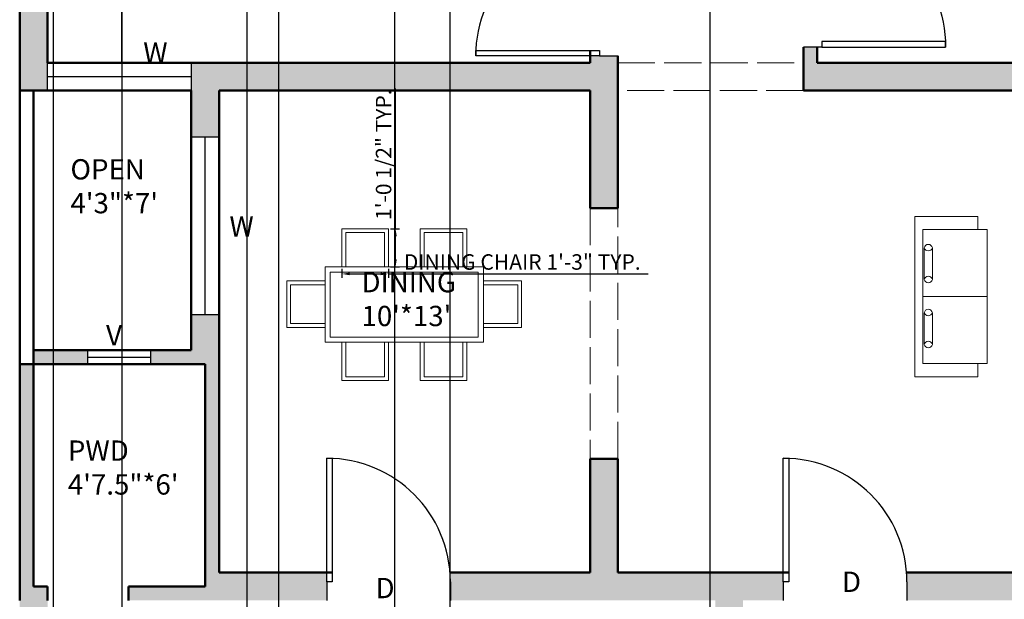
# Model space of a CAD drawing. Units: inches. Extents: x 2101 to 2663, y 1144 to 2069.
# Tile 2 of 4: x 2112 to 2431, y 1530 to 1718. Entities that reach past the tile are written whole.
import ezdxf

# ---------------------------------------------------------------- set-up
doc = ezdxf.new("R2010")
doc.units = ezdxf.units.IN
doc.linetypes.add('ACAD_ISO02W100', pattern=[15, 12, -3])
for name, color, linetype, lineweight in [('A-ANNO-DIMS', 2, 'Continuous', 18), ('A-ANNO-TEXT', 7, 'Continuous', 18), ('A-AREA-IDEN', 7, 'Continuous', 25), ('A-FLOR-CASE', 142, 'Continuous', 25), ('A-WALL-OVHD', 240, 'ACAD_ISO02W100', 18), ('A-WALL-PATT', 240, 'Continuous', 13), ('door', 52, 'Continuous', 25), ('fur', 142, 'Continuous', 18), ('wall', 240, 'Continuous', 50), ('win', 150, 'Continuous', 25)]:
    doc.layers.add(name, color=color, linetype=linetype, lineweight=lineweight)
doc.styles.get("Standard").update_dxf_attribs({"font": 'arial.ttf'})
doc.dimstyles.new('ISO-25', dxfattribs={"dimtxt": 5, "dimasz": 2.5, "dimexe": 1.25, "dimexo": 0.625, "dimtad": 1, "dimdec": 0, "dimlunit": 4, "dimtxsty": 'Standard', "dimcen": 2.5, "dimadec": 0, "dimazin": 0, "dimtfac": 1, "dimtdec": 0, "dimtmove": 0, "dimatfit": 3, "dimfxl": 1, "dimarcsym": 0})

# ---------------------------------------------------------------- blocks, each defined once
blk = doc.blocks.new('*U2')
for p, q in [((0, 0), (0, -6)), ((40, 0), (40, -6))]:
    blk.add_line(p, q)
blk.add_lwpolyline([(0, 0), (0, 40), (1.75, 40), (1.75, 0)], close=True)
blk.add_arc((0, 0), 40, 0, 90)
blk = doc.blocks.new('SOFA-TWO-SEAT')
for p, q in [((-8.65, 21.68), (-8.65, 25.93)), ((-8.65, 25.93), (11.73, 25.93)), ((11.73, 25.93), (11.73, -25.93)), ((-11.73, -0.01), (9.09, -0.01)), ((-8.65, -25.93), (-8.65, -21.7)), ((11.73, -25.93), (-8.65, -25.93))]:
    blk.add_line(p, q)
blk.add_lwpolyline([(9.09, 21.68), (-11.73, 21.68), (-11.73, -21.7), (9.09, -21.7)], close=True)
for points in [[(6.04, 5.2), (6.04, 15.47)], [(8.66, 15.47), (8.66, 5.2)], [(6.04, -15.8), (6.04, -5.54)], [(8.66, -5.54), (8.66, -15.8)]]:
    blk.add_lwpolyline(points)
for centre, radius, start, end in [((7.35, 15.19), 1.34, 11.9211, 168.0789), ((7.35, 15.75), 1.34, 191.8934, 348.1066), ((7.35, 4.81), 1.37, 16.4476, 163.5524), ((7.35, 5.4), 1.33, 188.6987, 351.3013), ((7.35, -5.81), 1.34, 11.9211, 168.0789), ((7.35, -5.26), 1.34, 191.8934, 348.1066), ((7.35, -16.19), 1.37, 16.4476, 163.5524), ((7.35, -15.6), 1.33, 188.6987, 351.3013)]:
    blk.add_arc(centre, radius, start, end)
blk = doc.blocks.new('CHAIR-DINING')
for p, q in [((-7.55, -6.18), (-7.55, 6.18)), ((-7.55, 6.18), (7.55, 6.18)), ((7.55, 6.18), (7.55, -6.18))]:
    blk.add_line(p, q)
blk.add_lwpolyline([(-6.25, -6.18), (6.27, -6.18), (6.27, 5), (-6.25, 5)], close=True)
blk = doc.blocks.new('*D25')
at = {"layer": 'A-ANNO-DIMS', "color": 0, "lineweight": -2, "transparency": 16777216}
for p, q in [((2216.58, 1636.95), (2216.58, 1634.06)), ((2219.08, 1635.31), (2229.18, 1635.31)), ((2231.68, 1636.95), (2231.68, 1634.06)), ((2231.68, 1635.31), (2315.72, 1635.31))]:
    blk.add_line(p, q, dxfattribs=at)
at = {"layer": 'A-ANNO-DIMS', "color": 0, "lineweight": 100, "transparency": 16777216}
for points in [[(2219.08, 1635.73), (2219.08, 1634.9), (2216.58, 1635.31)], [(2229.18, 1635.73), (2229.18, 1634.9), (2231.68, 1635.31)]]:
    blk.add_solid(points, dxfattribs=at)
at = {"layer": 'Defpoints', "color": 0, "lineweight": 100, "transparency": 16777216}
for p in [(2216.58, 1637.58), (2231.68, 1637.58), (2231.68, 1635.31)]:
    blk.add_point(p, dxfattribs=at)
at = {"layer": 'A-ANNO-DIMS', "color": 0, "transparency": 16777216, "insert": (2274.95, 1638.52), "char_height": 5, "attachment_point": 5}
blk.add_mtext('DINING CHAIR 1\'-3" TYP.', dxfattribs=at)
blk = doc.blocks.new('*D26')
at = {"layer": 'A-ANNO-DIMS', "color": 0, "lineweight": -2, "transparency": 16777216}
for p, q in [((2233.95, 1649.94), (2233.95, 1695.35)), ((2232.31, 1649.94), (2235.2, 1649.94)), ((2233.95, 1640.08), (2233.95, 1647.44)), ((2232.31, 1637.58), (2235.2, 1637.58))]:
    blk.add_line(p, q, dxfattribs=at)
at = {"layer": 'A-ANNO-DIMS', "color": 0, "lineweight": 100, "transparency": 16777216}
for points in [[(2233.53, 1647.44), (2234.37, 1647.44), (2233.95, 1649.94)], [(2233.53, 1640.08), (2234.37, 1640.08), (2233.95, 1637.58)]]:
    blk.add_solid(points, dxfattribs=at)
at = {"layer": 'Defpoints', "color": 0, "lineweight": 100, "transparency": 16777216}
for p in [(2231.68, 1649.94), (2233.95, 1649.94), (2231.68, 1637.58)]:
    blk.add_point(p, dxfattribs=at)
at = {"layer": 'A-ANNO-DIMS', "color": 0, "transparency": 16777216, "insert": (2230.74, 1673.89), "char_height": 5, "attachment_point": 5, "rotation": 90}
blk.add_mtext('1\'-0 1/2" TYP.', dxfattribs=at)
blk = doc.blocks.new('*D29')
at = {"layer": 'A-ANNO-DIMS', "color": 0, "lineweight": -2, "transparency": 16777216}
for p, q in [((2121.39, 1704.28), (2121.39, 2049.05)), ((2145.39, 1704.28), (2145.39, 2049.05)), ((2123.89, 2047.8), (2142.89, 2047.8))]:
    blk.add_line(p, q, dxfattribs=at)
at = {"layer": 'A-ANNO-DIMS', "color": 0, "lineweight": 100, "transparency": 16777216}
for points in [[(2123.89, 2048.22), (2123.89, 2047.38), (2121.39, 2047.8)], [(2142.89, 2048.22), (2142.89, 2047.38), (2145.39, 2047.8)]]:
    blk.add_solid(points, dxfattribs=at)
at = {"layer": 'Defpoints', "color": 0, "lineweight": 100, "transparency": 16777216}
for p in [(2145.39, 2047.8), (2121.39, 1703.65), (2145.39, 1703.65)]:
    blk.add_point(p, dxfattribs=at)
at = {"layer": 'A-ANNO-DIMS', "color": 0, "transparency": 16777216, "insert": (2133.39, 2050.98), "char_height": 5, "attachment_point": 5}
blk.add_mtext('2\'-0"', dxfattribs=at)
blk = doc.blocks.new('*D31')
at = {"layer": 'A-ANNO-DIMS', "color": 0, "lineweight": -2, "transparency": 16777216}
for p, q in [((2196.07, 1776.74), (2196.07, 1146.75)), ((2233.58, 1776.74), (2233.58, 1146.75)), ((2198.57, 1148), (2231.08, 1148))]:
    blk.add_line(p, q, dxfattribs=at)
at = {"layer": 'A-ANNO-DIMS', "color": 0, "lineweight": 100, "transparency": 16777216}
for points in [[(2198.57, 1148.42), (2198.57, 1147.58), (2196.07, 1148)], [(2231.08, 1148.42), (2231.08, 1147.58), (2233.58, 1148)]]:
    blk.add_solid(points, dxfattribs=at)
at = {"layer": 'Defpoints', "color": 0, "lineweight": 100, "transparency": 16777216}
for p in [(2196.07, 1777.37), (2233.58, 1777.37), (2233.58, 1148)]:
    blk.add_point(p, dxfattribs=at)
at = {"layer": 'A-ANNO-DIMS', "color": 0, "transparency": 16777216, "insert": (2214.83, 1151.21), "char_height": 5, "attachment_point": 5}
blk.add_mtext('3\'-1 1/2"', dxfattribs=at)
blk = doc.blocks.new('*D32')
at = {"layer": 'A-ANNO-DIMS', "color": 0, "lineweight": -2, "transparency": 16777216}
for p, q in [((2123.19, 1725.57), (2123.19, 1146.75)), ((2145.39, 1725.57), (2145.39, 1146.75)), ((2125.69, 1148), (2142.89, 1148))]:
    blk.add_line(p, q, dxfattribs=at)
at = {"layer": 'A-ANNO-DIMS', "color": 0, "lineweight": 100, "transparency": 16777216}
for points in [[(2125.69, 1148.42), (2125.69, 1147.58), (2123.19, 1148)], [(2142.89, 1148.42), (2142.89, 1147.58), (2145.39, 1148)]]:
    blk.add_solid(points, dxfattribs=at)
at = {"layer": 'Defpoints', "color": 0, "lineweight": 100, "transparency": 16777216}
for p in [(2123.19, 1726.19), (2145.39, 1726.19), (2145.39, 1148)]:
    blk.add_point(p, dxfattribs=at)
at = {"layer": 'A-ANNO-DIMS', "color": 0, "transparency": 16777216, "insert": (2134.29, 1151.18), "char_height": 5, "attachment_point": 5}
blk.add_mtext('1\'-10"', dxfattribs=at)
blk = doc.blocks.new('*D34')
at = {"layer": 'A-ANNO-DIMS', "color": 0, "lineweight": -2, "transparency": 16777216}
for p, q in [((2185.89, 1947.53), (2185.89, 1146.75)), ((2251.48, 1947.53), (2251.48, 1146.75)), ((2188.39, 1148), (2248.98, 1148))]:
    blk.add_line(p, q, dxfattribs=at)
at = {"layer": 'A-ANNO-DIMS', "color": 0, "lineweight": 100, "transparency": 16777216}
for points in [[(2188.39, 1148.42), (2188.39, 1147.58), (2185.89, 1148)], [(2248.98, 1148.42), (2248.98, 1147.58), (2251.48, 1148)]]:
    blk.add_solid(points, dxfattribs=at)
at = {"layer": 'Defpoints', "color": 0, "lineweight": 100, "transparency": 16777216}
for p in [(2185.89, 1948.15), (2251.48, 1948.15), (2251.48, 1148)]:
    blk.add_point(p, dxfattribs=at)
at = {"layer": 'A-ANNO-DIMS', "color": 0, "transparency": 16777216, "insert": (2218.69, 1151.21), "char_height": 5, "attachment_point": 5}
blk.add_mtext('5\'-5 1/2"', dxfattribs=at)
blk = doc.blocks.new('*D35')
at = {"layer": 'A-ANNO-DIMS', "color": 0, "lineweight": -2, "transparency": 16777216}
for p, q in [((2251.48, 1947.53), (2251.48, 1146.75)), ((2335.68, 1947.53), (2335.68, 1146.75)), ((2253.98, 1148), (2333.18, 1148))]:
    blk.add_line(p, q, dxfattribs=at)
at = {"layer": 'A-ANNO-DIMS', "color": 0, "lineweight": 100, "transparency": 16777216}
for points in [[(2253.98, 1148.42), (2253.98, 1147.58), (2251.48, 1148)], [(2333.18, 1148.42), (2333.18, 1147.58), (2335.68, 1148)]]:
    blk.add_solid(points, dxfattribs=at)
at = {"layer": 'Defpoints', "color": 0, "lineweight": 100, "transparency": 16777216}
for p in [(2251.48, 1948.15), (2335.68, 1948.15), (2335.68, 1148)]:
    blk.add_point(p, dxfattribs=at)
at = {"layer": 'A-ANNO-DIMS', "color": 0, "transparency": 16777216, "insert": (2293.58, 1151.18), "char_height": 5, "attachment_point": 5}
blk.add_mtext('7\'-0"', dxfattribs=at)

msp = doc.modelspace()

# ---------------------------------------------------------------- hatches: boundary and pattern name
at = {"layer": 'A-WALL-PATT'}
h = msp.add_hatch(color=256, dxfattribs=at)
h.dxf.hatch_style = 1
h.paths.add_polyline_path([(2190.39, 2003.65), (2185.89, 2003.65), (2112.39, 2003.65), (2112.39, 1882.15), (2112.39, 1799.65), (2112.39, 1694.65), (2121.39, 1694.65), (2121.39, 1703.65), (2121.39, 1799.65), (2121.39, 1804.15), (2121.39, 1882.15), (2145.24, 1882.15), (2145.24, 1886.65), (2121.39, 1886.65), (2121.39, 1917.6), (2121.39, 1994.65), (2181.39, 1994.65), (2181.39, 1990.84), (2190.39, 1990.84), (2190.39, 1999.15)])
h.paths.add_polyline_path([(2185.89, 1843.15), (2181.39, 1843.15), (2181.39, 1804.15), (2185.89, 1804.15)], flags=17)
h.paths.add_polyline_path([(2185.89, 1948.15), (2251.48, 1948.15), (2251.48, 1957.15), (2190.39, 1957.15), (2190.39, 1968.84), (2181.39, 1968.84), (2181.39, 1968.14), (2181.39, 1886.65), (2178.82, 1886.65), (2178.82, 1882.15), (2181.39, 1882.15), (2181.39, 1876.17), (2185.89, 1876.17), (2185.89, 1882.15)])
h.paths.add_polyline_path([(2482.89, 1957.15), (2335.68, 1957.15), (2335.68, 1948.15), (2365.89, 1948.15), (2482.89, 1948.15)])
h.paths.add_polyline_path([(2539.89, 1957.15), (2515.98, 1957.15), (2507.18, 1957.15), (2507.18, 1948.15), (2530.89, 1948.15), (2530.89, 1864.15), (2530.89, 1859.65), (2539.89, 1859.65), (2539.89, 1864.15), (2539.89, 1883.02)])
h.paths.add_polyline_path([(2539.89, 1859.65), (2530.89, 1859.65), (2530.89, 1819.07), (2539.89, 1819.07)])
h.paths.add_polyline_path([(2530.89, 1864.15), (2434.89, 1864.15), (2434.89, 1859.65), (2530.89, 1859.65)])
h.paths.add_polyline_path([(2388.94, 1864.15), (2370.39, 1864.15), (2370.39, 1859.65), (2388.94, 1859.65)])
h.paths.add_polyline_path([(2434.89, 1864.15), (2434.89, 1870.19), (2430.39, 1870.19), (2430.39, 1864.15), (2424.15, 1864.15), (2424.15, 1859.65), (2434.89, 1859.65)])
h.paths.add_polyline_path([(2434.89, 1948.15), (2430.39, 1948.15), (2430.39, 1910.19), (2434.89, 1910.19)])
h.paths.add_polyline_path([(2370.39, 1948.15), (2365.89, 1948.15), (2365.89, 1804.15), (2365.89, 1795.15), (2370.39, 1795.15), (2370.39, 1859.65), (2370.39, 1864.15)])
h.paths.add_polyline_path([(2539.89, 1747.47), (2530.89, 1747.47), (2530.89, 1703.65), (2370.39, 1703.65), (2370.39, 1708.72), (2365.89, 1708.72), (2365.89, 1694.65), (2539.89, 1694.65)])
h.paths.add_polyline_path([(2539.89, 1694.65), (2530.89, 1694.65), (2530.89, 1656.23), (2539.89, 1656.23)])
h = msp.add_hatch(color=256, dxfattribs=at)
h.dxf.hatch_style = 1
h.paths.add_polyline_path([(2305.89, 1705.85), (2299.89, 1705.85), (2296.89, 1705.85), (2296.89, 1703.65), (2167.89, 1703.65), (2167.89, 1694.65), (2305.89, 1694.65)])
h.paths.add_polyline_path([(2305.89, 1804.15), (2121.39, 1804.15), (2121.39, 1799.65), (2296.89, 1799.65), (2296.89, 1775.65), (2296.89, 1745.74, -0.01877), (2299.89, 1745.85), (2305.89, 1745.85)])
h.paths.add_polyline_path([(2319.05, 1801.15, -0.01877), (2319.16, 1804.15), (2305.89, 1804.15), (2305.89, 1795.15), (2319.05, 1795.15)])
h.paths.add_polyline_path([(2365.89, 1804.15), (2359.05, 1804.15), (2359.05, 1801.15), (2359.05, 1795.15), (2365.89, 1795.15)])
h.paths.add_polyline_path([(2370.39, 1795.15), (2365.89, 1795.15), (2365.89, 1748.72), (2370.39, 1748.72)])
h.paths.add_polyline_path([(2305.89, 1694.65), (2296.89, 1694.65), (2296.89, 1656.63), (2305.89, 1656.63)])
h.paths.add_polyline_path([(2176.89, 1694.65), (2167.89, 1694.65), (2167.89, 1679.51), (2176.89, 1679.51)])
h.paths.add_polyline_path([(2134.3, 1610.65), (2116.89, 1610.65), (2116.89, 1606.15), (2134.3, 1606.15)])
h.paths.add_polyline_path([(2176.89, 1622.19), (2167.89, 1622.19), (2167.89, 1610.65), (2154.79, 1610.65), (2154.79, 1606.15), (2176.89, 1606.15)])
h.paths.add_polyline_path([(2176.89, 1606.15), (2172.39, 1606.15), (2172.39, 1534.15), (2147.63, 1534.15), (2147.63, 1529.65), (2176.89, 1529.65)])
h.paths.add_polyline_path([(2211.7, 1535.65), (2211.7, 1538.65), (2176.89, 1538.65), (2176.89, 1529.65), (2211.7, 1529.65)])
h.paths.add_polyline_path([(2116.89, 1606.15), (2112.39, 1606.15), (2112.39, 1529.65), (2121.39, 1529.65), (2121.39, 1534.15), (2116.89, 1534.15)])
h.paths.add_polyline_path([(2121.39, 1529.65), (2112.39, 1529.65), (2112.39, 1485), (2121.39, 1485)])
h.paths.add_polyline_path([(2359.39, 1535.65), (2359.39, 1538.65), (2314.89, 1538.65), (2251.59, 1538.65, -0.01877), (2251.7, 1535.65), (2251.7, 1529.65), (2359.39, 1529.65)])
h.paths.add_polyline_path([(2305.89, 1575.46), (2296.89, 1575.46), (2296.89, 1538.65), (2305.89, 1538.65)])
h.paths.add_polyline_path([(2539.89, 1584.63), (2530.89, 1584.63), (2530.89, 1538.65), (2399.28, 1538.65, -0.01877), (2399.39, 1535.65), (2399.39, 1529.65), (2539.89, 1529.65)])
h.paths.add_polyline_path([(2346.39, 1370.88), (2340.39, 1370.88), (2337.39, 1370.88), (2337.39, 1361.65), (2308.27, 1361.65), (2308.27, 1352.65), (2346.39, 1352.65)])
h.paths.add_polyline_path([(2168.45, 1361.65), (2121.39, 1361.65), (2121.39, 1417.42), (2112.39, 1417.42), (2112.39, 1352.65), (2168.45, 1352.65)])
h.paths.add_polyline_path([(2346.39, 1529.65), (2337.39, 1529.65), (2337.39, 1414.47), (2337.39, 1410.77, -0.01877), (2340.39, 1410.88), (2346.39, 1410.88), (2346.39, 1414.47)])
h.paths.add_polyline_path([(2592.39, 1433.97), (2583.39, 1433.97), (2583.39, 1292.97), (2592.39, 1292.97)])
h.paths.add_polyline_path([(2592.39, 1204.95), (2583.39, 1204.95), (2583.39, 1196.65), (2578.02, 1196.65), (2578.02, 1192.15), (2592.39, 1192.15)])
h.paths.add_polyline_path([(2583.39, 1204.95), (2578.02, 1204.95), (2578.02, 1196.65), (2583.39, 1196.65)], flags=17)
h.paths.add_polyline_path([(2382.99, 1204.95), (2368.62, 1204.95), (2368.62, 1196.65), (2382.99, 1196.65)])
h.paths.add_polyline_path([(2382.99, 1196.65), (2368.62, 1196.65), (2368.62, 1192.15), (2382.99, 1192.15)])
h.paths.add_polyline_path([(2490.54, 1433.65), (2490.54, 1424.65), (2539.89, 1424.65), (2539.89, 1433.97), (2539.89, 1529.65), (2530.89, 1529.65), (2530.89, 1433.65)])
h.paths.add_polyline_path([(2438.35, 1424.65), (2438.35, 1433.65), (2400.84, 1433.65), (2400.84, 1424.65)])

# ---------------------------------------------------------------- linework, layer by layer
at = {"layer": 'A-FLOR-CASE'}
for p, q in [((2145.39, 1703.65), (2145.39, 1775.65)), ((2121.39, 1703.65), (2145.39, 1703.65))]:
    msp.add_line(p, q, dxfattribs=at)
at = {"layer": 'A-WALL-OVHD'}
for points in [[(2305.89, 1703.65), (2365.89, 1703.65), (2365.89, 1694.65), (2305.89, 1694.65)], [(2296.89, 1575.46), (2305.89, 1575.46), (2305.89, 1656.63), (2296.89, 1656.63)]]:
    msp.add_lwpolyline(points, close=True, dxfattribs=at)
at = {"layer": 'fur'}
for points in [[(2211.21, 1637.58), (2262.39, 1637.58), (2262.39, 1613.2), (2211.21, 1613.2)], [(2212.86, 1635.93), (2260.74, 1635.93), (2260.74, 1614.85), (2212.86, 1614.85)]]:
    msp.add_lwpolyline(points, close=True, dxfattribs=at)
at = {"layer": 'wall'}
for p, q in [((2112.39, 1694.65), (2112.39, 1799.65)), ((2121.39, 1703.65), (2121.39, 1799.65)), ((2296.89, 1707.6), (2296.89, 1703.65)), ((2365.89, 1708.72), (2365.89, 1694.65)), ((2370.39, 1708.72), (2370.39, 1703.65)), ((2305.89, 1705.85), (2305.89, 1694.65)), ((2296.89, 1703.65), (2121.39, 1703.65)), ((2370.39, 1703.65), (2530.89, 1703.65)), ((2112.39, 1694.65), (2112.39, 1606.15)), ((2112.39, 1606.15), (2112.39, 1694.65)), ((2167.89, 1694.65), (2112.39, 1694.65)), ((2116.89, 1694.65), (2116.89, 1622.65)), ((2116.89, 1694.65), (2116.89, 1610.65)), ((2116.89, 1610.65), (2116.89, 1694.65)), ((2167.89, 1694.65), (2167.89, 1610.65)), ((2296.89, 1694.65), (2176.89, 1694.65)), ((2176.89, 1694.65), (2176.89, 1606.15)), ((2176.89, 1694.65), (2296.89, 1694.65)), ((2296.89, 1694.65), (2296.89, 1656.63)), ((2305.89, 1694.65), (2305.89, 1656.63)), ((2365.89, 1694.65), (2530.89, 1694.65)), ((2296.89, 1656.63), (2305.89, 1656.63)), ((2116.89, 1610.65), (2167.89, 1610.65)), ((2116.89, 1610.65), (2116.89, 1606.15)), ((2112.39, 1606.15), (2172.39, 1606.15)), ((2112.39, 1606.15), (2112.39, 1529.65)), ((2116.89, 1606.15), (2116.89, 1534.15)), ((2172.39, 1534.15), (2172.39, 1606.15)), ((2176.89, 1538.65), (2176.89, 1606.15)), ((2296.89, 1575.46), (2305.89, 1575.46)), ((2296.89, 1575.46), (2296.89, 1538.65)), ((2305.89, 1575.46), (2305.89, 1538.65)), ((2176.89, 1538.65), (2213.45, 1538.65)), ((2213.45, 1538.65), (2176.89, 1538.65)), ((2296.89, 1538.65), (2251.59, 1538.65)), ((2251.59, 1538.65), (2296.89, 1538.65)), ((2305.89, 1538.65), (2346.39, 1538.65)), ((2361.14, 1538.65), (2314.89, 1538.65)), ((2530.89, 1538.65), (2399.28, 1538.65)), ((2116.89, 1534.15), (2121.39, 1534.15)), ((2121.39, 1529.65), (2121.39, 1534.15)), ((2147.63, 1534.15), (2147.63, 1529.65)), ((2147.63, 1534.15), (2172.39, 1534.15))]:
    msp.add_line(p, q, dxfattribs=at)
at = {"layer": 'win'}
for p, q in [((2121.39, 1699.15), (2167.89, 1699.15)), ((2116.89, 1694.65), (2167.89, 1694.65)), ((2172.39, 1622.19), (2172.39, 1679.51)), ((2134.3, 1608.4), (2154.79, 1608.4))]:
    msp.add_line(p, q, dxfattribs=at)
for points in [[(2167.89, 1694.65), (2121.39, 1694.65), (2121.39, 1703.65), (2167.89, 1703.65)], [(2167.89, 1622.19), (2176.89, 1622.19), (2176.89, 1679.51), (2167.89, 1679.51)], [(2134.3, 1606.15), (2154.79, 1606.15), (2154.79, 1610.65), (2134.3, 1610.65)]]:
    msp.add_lwpolyline(points, close=True, dxfattribs=at)

# ---------------------------------------------------------------- block references
at = {"layer": 'door', "xscale": -1, "rotation": 270}
msp.add_blockref('*U2', (2371.89, 1708.72), dxfattribs=at)
at = {"layer": 'door', "rotation": 90}
msp.add_blockref('*U2', (2299.89, 1705.85), dxfattribs=at)
at = {"layer": 'door'}
for p in [(2211.7, 1535.65), (2359.39, 1535.65)]:
    msp.add_blockref('*U2', p, dxfattribs=at)
at = {"layer": 'fur'}
for name, p, rotation in [('SOFA-TWO-SEAT', (2413.64, 1627.95), 180), ('CHAIR-DINING', (2205.03, 1625.53), 89.99999999999785)]:
    msp.add_blockref(name, p, dxfattribs=dict(at, rotation=rotation))
for p in [(2224.13, 1643.76), (2249.45, 1643.76)]:
    msp.add_blockref('CHAIR-DINING', p, dxfattribs=at)
at = {"layer": 'fur', "extrusion": (0, 0, -1), "zscale": -1}
for p, rotation in [((-2268.57, 1625.53), 89.99999999999982), ((-2224.13, 1607.02), 180), ((-2249.45, 1607.02), 180)]:
    msp.add_blockref('CHAIR-DINING', p, dxfattribs=dict(at, rotation=rotation))

# ---------------------------------------------------------------- texts
at = {"layer": 'A-ANNO-TEXT', "char_height": 6.57, "attachment_point": 1}
for s, insert in [('W', (2152.36, 1710.22)), ('W', (2180.23, 1653.97)), ('V', (2140.33, 1618.74)), ('D', (2378.37, 1538.97)), ('D', (2227.49, 1536.95))]:
    msp.add_mtext_dynamic_manual_height_columns(s, width=76.8305, gutter_width=32.84, heights=[0], dxfattribs=dict(at, insert=insert))
at = {"layer": 'A-AREA-IDEN', "char_height": 6.568, "attachment_point": 1}
for s, insert in [('OPEN\\P4\'3"*7\'', (2128.81, 1672.44)), ("DINING\\P10'*13'", (2222.96, 1635.93)), ('PWD\\P4\'7.5"*6\'', (2127.97, 1581.42))]:
    msp.add_mtext_dynamic_manual_height_columns(s, width=76.8305, gutter_width=32.84, heights=[0], dxfattribs=dict(at, insert=insert))

# ---------------------------------------------------------------- dimensions: what is measured, and where the dimension line sits
at = {"layer": 'A-ANNO-DIMS'}
for base, p1, p2, picture, middle in [((2145.39, 2047.8), (2121.39, 1703.65), (2145.39, 1703.65), '*D29', (2133.39, 2050.98)), ((2251.48, 1148), (2185.89, 1948.15), (2251.48, 1948.15), '*D34', (2218.69, 1151.21)), ((2335.68, 1148), (2251.48, 1948.15), (2335.68, 1948.15), '*D35', (2293.58, 1151.18)), ((2233.58, 1148), (2196.07, 1777.37), (2233.58, 1777.37), '*D31', (2214.83, 1151.21)), ((2145.39, 1148), (2123.19, 1726.19), (2145.39, 1726.19), '*D32', (2134.29, 1151.18))]:
    dim = msp.add_linear_dim(base=base, p1=p1, p2=p2, dimstyle='ISO-25', override={"dimdec": 1, "dimlfac": 1, "dimrnd": 0, "dimzin": 1, "dimdsep": 46, "dimlunit": 4, "dimfrac": 2}, dxfattribs=at)
    dim.commit()
    dim.dimension.update_dxf_attribs({"geometry": picture, "text_midpoint": middle})
dim = msp.add_linear_dim(base=(2233.95, 1649.94), p1=(2231.68, 1637.58), p2=(2231.68, 1649.94), angle=90, text='<> TYP.', dimstyle='ISO-25', override={"dimdec": 1, "dimlfac": 1, "dimrnd": 0, "dimzin": 1, "dimdsep": 46, "dimlunit": 4, "dimfrac": 2}, dxfattribs=at)
dim.commit()
dim.dimension.update_dxf_attribs({"geometry": '*D26', "text_midpoint": (2230.74, 1673.89)})
dim = msp.add_linear_dim(base=(2231.68, 1635.31), p1=(2216.58, 1637.58), p2=(2231.68, 1637.58), text='DINING CHAIR <> TYP.', dimstyle='ISO-25', override={"dimdec": 1, "dimlfac": 1, "dimrnd": 0, "dimzin": 1, "dimdsep": 46, "dimlunit": 4, "dimfrac": 2}, dxfattribs=at)
dim.commit()
dim.dimension.update_dxf_attribs({"geometry": '*D25', "text_midpoint": (2274.95, 1638.52)})

doc.saveas('drawing.dxf')
